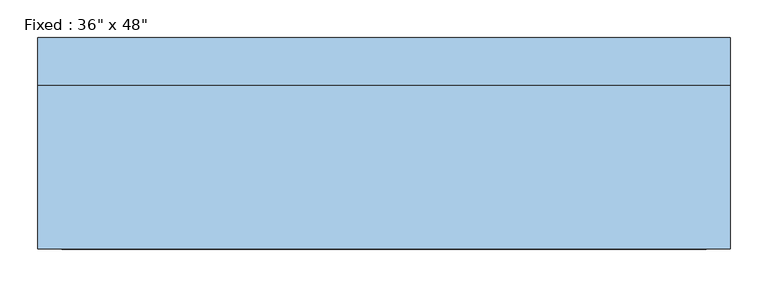
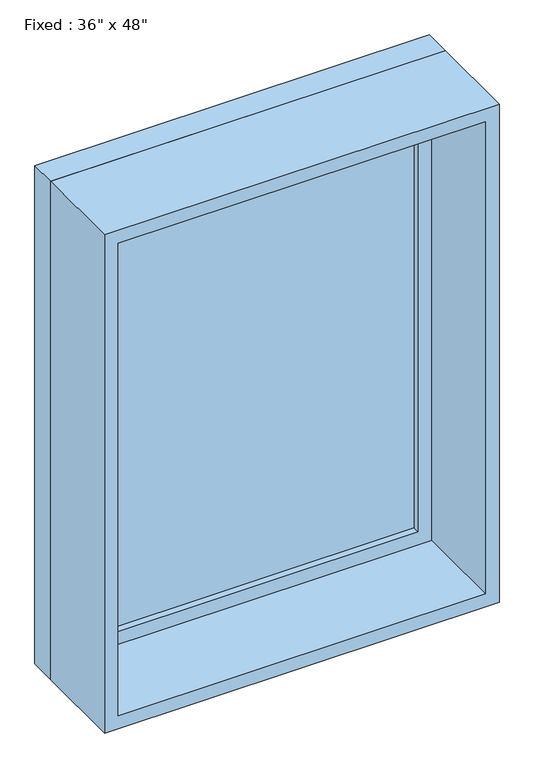
"""IFC4 building model written with IfcOpenShell, lengths in millimetres: window geometry."""

from ifc_helpers import new_model, si_unit, frame, origin, place, context, project, spatial, polyline, outline, extrude, source, transform, mapped, element, save


def window_60f40170(model_context):
    return source(origin(), model_context, "Body", "SweptSolid", [
        extrude(outline(polyline([(355.6, 92.075), (-431.8, 92.075), (-431.8, 104.775), (355.6, 104.775), (355.6, 92.075)])), frame((0.0, 0.0, 977.9), z_axis=(0.0, 0.0, 1.0), x_axis=(1.0, 0.0, 0.0)), (0.0, 0.0, 1.0), 1092.2),
        extrude(outline(polyline([(2114.55, -476.25), (933.45, -476.25), (933.45, 400.05), (2114.55, 400.05), (2114.55, -476.25)]), holes=[polyline([(2070.1, -431.8), (2070.1, 355.6), (977.9, 355.6), (977.9, -431.8), (2070.1, -431.8)])]), frame((0.0, 76.2, 0.0), z_axis=(0.0, 1.0, 0.0), x_axis=(0.0, 0.0, 1.0)), (0.0, 0.0, 1.0), 44.45),
        extrude(outline(polyline([(2133.6, -495.3), (914.4, -495.3), (914.4, 419.1), (2133.6, 419.1), (2133.6, -495.3)]), holes=[polyline([(2101.85, -463.55), (2101.85, 387.35), (946.15, 387.35), (946.15, -463.55), (2101.85, -463.55)])]), frame((0.0, -139.7, 0.0), z_axis=(0.0, 1.0, 0.0), x_axis=(0.0, 0.0, 1.0)), (0.0, 0.0, 1.0), 215.9),
        extrude(outline(polyline([(2133.6, 419.1), (2133.6, -495.3), (914.4, -495.3), (914.4, 419.1), (2133.6, 419.1)]), holes=[polyline([(2114.55, 400.05), (933.45, 400.05), (933.45, -476.25), (2114.55, -476.25), (2114.55, 400.05)])]), frame((0.0, 76.2, 0.0), z_axis=(0.0, 1.0, 0.0), x_axis=(0.0, 0.0, 1.0)), (0.0, 0.0, 1.0), 63.5),
    ])


if __name__ == "__main__":
    model = new_model("IFC4")
    model_context = context("Model", 3, world=origin())
    ifc_project = project(units=[si_unit("LENGTHUNIT", "METRE", prefix="MILLI")], contexts=[model_context])
    site = spatial("IfcSite", under=ifc_project)
    building = spatial("IfcBuilding", under=site)
    placement = place(None, origin())
    window_shape = window_60f40170(model_context)
    element("IfcWindow", 1, ObjectType="Fixed : 36\" x 48\"", at=placement, inside=building, context=model_context, shape_type="MappedRepresentation", body=[
        mapped(window_shape, transform((0.0, 0.0, 0.0), x_axis=(1.0, 0.0, 0.0), y_axis=(0.0, 1.0, 0.0), z_axis=(0.0, 0.0, 1.0))),
    ])
    save(model, "model.ifc")

# Revit data of these elements
# Type "Fixed : 36\" x 48\""
#   Type Mark = "1"
#   Construction Type Id = "GSP4R"
#   Assembly Code = "B2020100"
#   Analytic Construction = "1/8 in Pilkington single glazing"
#   Visual Light Transmittance = 0.9
#   Solar Heat Gain Coefficient = 0.78
#   Heat Transfer Coefficient (U) = 0.6496 BTU/(h·ft²·°F)
#   Height = 4' - 0"
#   Default Sill Height = 3' - 0"
#   Width = 3' - 0"
#   Window Inset = 0' - 0 3/4"
#   Define Thermal Properties by = 1
#   Define Thermal Properties by = 1
#   Glass Pane Material = Glass
#   Sash Material = Sash
#   Wall Closure = (empty or 0)
# Element 1 (IfcWindow, "Fixed : 36\" x 48\"")
#   Materials on its faces: "Sash", "Glass"
# Materials
#   "Glass": class "Glass", colour RGB 0 128 192, transparency 0.75, Description = "Soda Lime Glass", Cost = 0
#   "Sash": class "Wood", colour RGB 224 178 126, transparency 0, Cost = 0
